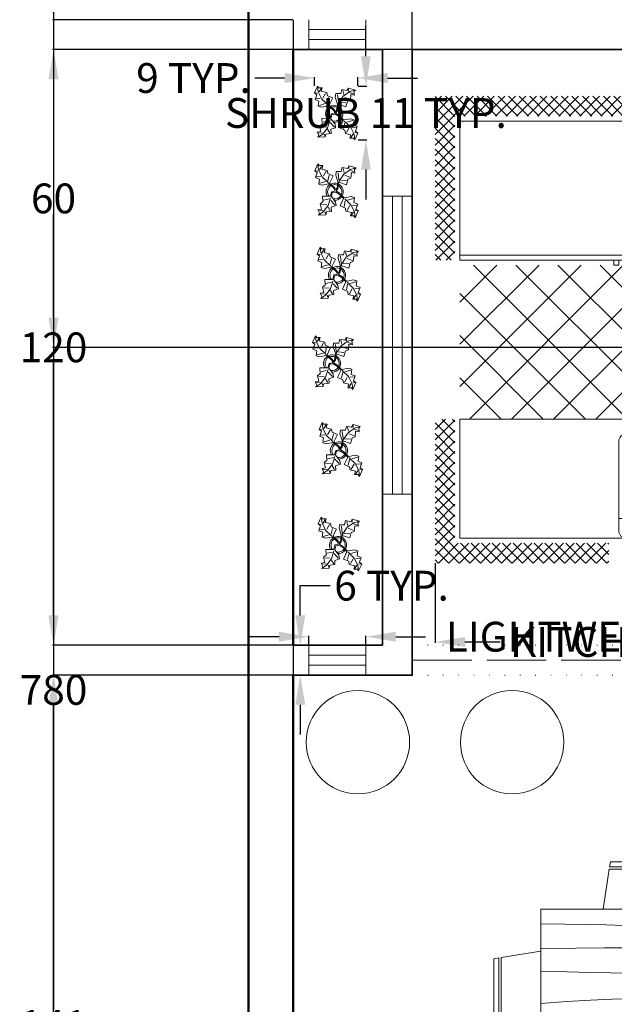
# Model space of a CAD drawing. Units: inches. Extents: x 823 to 1335, y 207 to 1074.
# Tile 3 of 6: x 823 to 943, y 577 to 776. Entities that reach past the tile are written whole.
import ezdxf

# ---------------------------------------------------------------- set-up
doc = ezdxf.new("R2010")
doc.units = ezdxf.units.IN
doc.header["$MEASUREMENT"] = 0
doc.linetypes.add('ACAD_ISO02W100', pattern=[15, 12, -3])
doc.linetypes.add('ACAD_ISO07W100', pattern=[3, 0, -3])
for name, color, linetype, lineweight in [('A-ANNO-DIMS', 2, 'Continuous', 18), ('A-GLAZ-HIDN', 211, 'ACAD_ISO02W100', 18), ('A-GLAZ-OVHD', 211, 'ACAD_ISO07W100', 18), ('furniture', 21, 'Continuous', 18), ('inner wall', 102, 'Continuous', 35), ('kitchen', 171, 'Continuous', 18), ('L-PLNT', 90, 'Continuous', 13), ('outer wall', 105, 'Continuous', 50), ('windows', 211, 'Continuous', 18)]:
    doc.layers.add(name, color=color, linetype=linetype, lineweight=lineweight)
doc.styles.get("Standard").update_dxf_attribs({"font": 'arial.ttf'})
doc.dimstyles.get("Standard").update_dxf_attribs({"dimtxt": 6, "dimasz": 6, "dimexe": 0.18, "dimexo": 0.0625, "dimgap": 0.09, "dimtad": 0, "dimtih": 1, "dimtoh": 1, "dimdec": 0, "dimzin": 0, "dimdsep": 46, "dimlunit": 3, "dimtxsty": 'Standard', "dimcen": 0.09, "dimadec": 0, "dimazin": 0, "dimtfac": 1, "dimtdec": 0, "dimtofl": 0, "dimtmove": 0, "dimatfit": 3, "dimfxl": 1, "dimtolj": 1, "dimtzin": 0, "dimarcsym": 0})

# ---------------------------------------------------------------- blocks, each defined once
blk = doc.blocks.new('Dining Set - 36 x 72 in.')
for p, q in [((-22.2343, 26.00059), (-23.4847, 17.99762)), ((-22.2304, 26), (-5.7608, 26)), ((-22, 27.5), (-22.1562, 26.50042)), ((-5.8416, 26.5), (-22.1534, 26.5)), ((-22, 27.5), (-6, 27.5)), ((-5.8437, 26.49966), (-6, 27.5)), ((-4.5152, 17.99762), (-5.7655, 25.99926)), ((5.7657, 26.00059), (4.5153, 17.99762)), ((5.7696, 26), (22.2392, 26)), ((6, 27.5), (5.8438, 26.50042)), ((22.1584, 26.5), (5.8466, 26.5)), ((6, 27.5), (22, 27.5)), ((22.1563, 26.49966), (22, 27.5)), ((23.4848, 17.99762), (22.2345, 25.99926)), ((36, 18), (-36, 18)), ((-36, 18), (-36, -18)), ((36, -18), (36, 18)), ((-45.5, 8), (-44.5004, 8.15617)), ((-45.5, 8), (-45.5, -8)), ((-44.5, -8.15843), (-44.5, 8.15338)), ((-44.0006, 8.23428), (-35.9976, 9.48474)), ((-44, 8.23041), (-44, -8.23915)), ((44.0006, 8.23428), (35.9976, 9.48474)), ((44, 8.23041), (44, -8.23915)), ((44.5, -8.15843), (44.5, 8.15338)), ((45.5, 8), (44.5005, 8.15617)), ((45.5, 8), (45.5, -8)), ((-44.4997, -8.15631), (-45.5, -8)), ((-35.9976, -9.48476), (-43.9993, -8.2345)), ((35.9976, -9.48476), (43.9993, -8.2345)), ((44.4997, -8.15631), (45.5, -8)), ((-36, -18), (36, -18)), ((-22.2343, -26.0006), (-23.4847, -17.99762)), ((-4.5152, -17.99762), (-5.7655, -25.99928)), ((5.7657, -26.0006), (4.5153, -17.99762)), ((23.4848, -17.99762), (22.2345, -25.99928)), ((-22.2304, -26), (-5.7608, -26)), ((-22, -27.5), (-22.1562, -26.50044)), ((-5.8416, -26.5), (-22.1534, -26.5)), ((-22, -27.5), (-6, -27.5)), ((-5.8437, -26.49967), (-6, -27.5)), ((5.7696, -26), (22.2392, -26)), ((6, -27.5), (5.8438, -26.50044)), ((22.1584, -26.5), (5.8466, -26.5)), ((6, -27.5), (22, -27.5)), ((22.1563, -26.49967), (22, -27.5))]:
    blk.add_line(p, q)
for points in [[(-36, 15), (-31.1772, 14.97754), (-26.8079, 14.91406), (-22.8538, 14.81543), (-19.276, 14.6875), (-16.0362, 14.53613), (-13.0957, 14.36718), (-10.4159, 14.18652), (-7.9583, 14), (-5.6904, 13.81315), (-3.6035, 13.63021), (-1.6954, 13.45508), (0.0365, 13.29166), (1.5945, 13.14388), (2.9811, 13.01562), (4.1988, 12.9108), (5.25, 12.83333), (6.1393, 12.78613), (6.8802, 12.76823), (7.4883, 12.77767), (7.9792, 12.8125), (8.3685, 12.87077), (8.6719, 12.95052), (8.9049, 13.0498), (9.0833, 13.16666), (9.2205, 13.29899), (9.3216, 13.44401), (9.3895, 13.59879), (9.4271, 13.76041), (9.4373, 13.92594), (9.4232, 14.09245), (9.3875, 14.257), (9.3333, 14.41666), (9.2638, 14.56917), (9.1836, 14.71484), (9.0975, 14.85465), (9.0104, 14.98958), (8.9272, 15.1206), (8.8529, 15.2487), (8.7922, 15.37483), (8.75, 15.5), (8.7305, 15.62467), (8.7344, 15.74739), (8.7617, 15.86621), (8.8125, 15.97916), (8.8867, 16.08431), (8.9844, 16.17968), (9.1055, 16.26334), (9.25, 16.33333), (9.4189, 16.38802), (9.6172, 16.42708), (9.8506, 16.45052), (10.125, 16.45833), (10.4463, 16.45052), (10.8203, 16.42708), (11.2529, 16.38802), (11.75, 16.33333), (12.3184, 16.26318), (12.9694, 16.17838), (13.7151, 16.07991), (14.5677, 15.96875), (15.5395, 15.84586), (16.6426, 15.71224), (17.8893, 15.56884), (19.2917, 15.41666), (20.859, 15.25667), (22.5879, 15.08984), (24.4721, 14.91715), (26.5052, 14.73958), (28.6809, 14.5581), (30.9929, 14.3737), (33.4347, 14.18733), (36, 14)], [(-36, 10), (-28.9766, 10.14274), (-23.1725, 10.20442), (-18.4241, 10.19775), (-14.5677, 10.13541), (-11.4399, 10.03011), (-8.877, 9.89453), (-6.7154, 9.74137), (-4.7917, 9.58333), (-2.9698, 9.43082), (-1.2246, 9.28515), (0.4415, 9.14534), (2.026, 9.01041), (3.5266, 8.87939), (4.9408, 8.7513), (6.266, 8.62516), (7.5, 8.5), (8.6411, 8.37549), (9.6914, 8.2539), (10.6538, 8.13818), (11.5312, 8.03125), (12.3267, 7.93603), (13.043, 7.85547), (13.6831, 7.79248), (14.25, 7.75), (14.7471, 7.7303), (15.1797, 7.73307), (15.5537, 7.75732), (15.875, 7.80208), (16.1494, 7.86637), (16.3828, 7.94922), (16.5811, 8.04964), (16.75, 8.16666), (16.8944, 8.29915), (17.0143, 8.44531), (17.1089, 8.60319), (17.1771, 8.77083), (17.218, 8.94629), (17.2305, 9.1276), (17.2137, 9.31282), (17.1667, 9.5), (17.0895, 9.6875), (16.987, 9.875), (16.8649, 10.0625), (16.7292, 10.25), (16.5856, 10.4375), (16.4401, 10.625), (16.2985, 10.8125), (16.1667, 11), (16.05, 11.18733), (15.9518, 11.3737), (15.8752, 11.5581), (15.8229, 11.73958), (15.798, 11.91715), (15.8034, 12.08984), (15.842, 12.25667), (15.9167, 12.41666), (16.0295, 12.56836), (16.1784, 12.70833), (16.3605, 12.83268), (16.5729, 12.9375), (16.8127, 13.01888), (17.0768, 13.07291), (17.3625, 13.0957), (17.6667, 13.08333), (17.9894, 13.03312), (18.3418, 12.94726), (18.7382, 12.82918), (19.1927, 12.68229), (19.7195, 12.51001), (20.3327, 12.31575), (21.0465, 12.10294), (21.875, 11.875), (22.8357, 11.63354), (23.959, 11.37304), (25.2786, 11.08618), (26.8282, 10.76562), (28.6414, 10.40405), (30.752, 9.99414), (33.1936, 9.52856), (36, 9)], [(-36, 5.5), (-30.7157, 5.3348), (-26.069, 5.20963), (-21.9946, 5.11767), (-18.4271, 5.05208), (-15.3009, 5.00602), (-12.5508, 4.97265), (-10.1112, 4.94515), (-7.9167, 4.91666), (-5.909, 4.88167), (-4.0586, 4.83984), (-2.3429, 4.79215), (-0.7396, 4.73958), (0.7739, 4.6831), (2.22, 4.6237), (3.6213, 4.56233), (5, 4.5), (6.373, 4.43782), (7.7344, 4.3776), (9.0723, 4.32129), (10.375, 4.27083), (11.6309, 4.22819), (12.8281, 4.19531), (13.9551, 4.17415), (15, 4.16666), (15.954, 4.17448), (16.819, 4.19791), (17.6001, 4.23698), (18.3021, 4.29166), (18.9299, 4.36198), (19.4883, 4.44791), (19.9823, 4.54948), (20.4167, 4.66666), (20.7969, 4.79899), (21.1302, 4.94401), (21.4245, 5.09879), (21.6875, 5.26041), (21.9271, 5.42594), (22.1511, 5.59245), (22.3672, 5.757), (22.5834, 5.91666), (22.8065, 6.06868), (23.0404, 6.21093), (23.2879, 6.34147), (23.5521, 6.45833), (23.8358, 6.55957), (24.142, 6.64323), (24.4735, 6.70735), (24.8334, 6.75), (25.2235, 6.76969), (25.642, 6.76692), (26.0858, 6.74267), (26.5521, 6.69791), (27.0379, 6.63362), (27.5404, 6.55078), (28.0565, 6.45036), (28.5834, 6.33333), (29.1242, 6.19987), (29.7071, 6.04687), (30.3661, 5.87044), (31.1354, 5.66666), (32.0493, 5.43164), (33.142, 5.16146), (34.4475, 4.85221), (36, 4.5)], [(-36, -1), (-30.7915, -0.6591), (-26.0195, -0.38216), (-21.6519, -0.16284), (-17.6563, 0.00521), (-14.0005, 0.12833), (-10.6523, 0.21289), (-7.5796, 0.26522), (-4.75, 0.29166), (-2.134, 0.29793), (0.2878, 0.28711), (2.5317, 0.26163), (4.6146, 0.22396), (6.5529, 0.17651), (8.3633, 0.12174), (10.0623, 0.06209), (11.6667, 0), (13.1899, -0.06201), (14.6341, -0.1211), (15.9982, -0.17432), (17.2813, -0.21875), (18.4823, -0.25147), (19.6003, -0.26953), (20.6343, -0.27002), (21.5834, -0.25), (22.4481, -0.20768), (23.2357, -0.14584), (23.9549, -0.06836), (24.6146, 0.02083), (25.2235, 0.11784), (25.7904, 0.21875), (26.3241, 0.31966), (26.8334, 0.41666), (27.3265, 0.50618), (27.8099, 0.58593), (28.2894, 0.65397), (28.7709, 0.70833), (29.2601, 0.74707), (29.763, 0.76823), (30.2855, 0.76985), (30.8334, 0.75), (31.4088, 0.70784), (31.9994, 0.64713), (32.589, 0.57275), (33.1615, 0.48958), (33.7008, 0.4025), (34.1908, 0.3164), (34.6153, 0.23616), (34.9584, 0.16666), (35.2099, 0.11165), (35.3848, 0.07031), (35.504, 0.04069), (35.5886, 0.02083), (35.6594, 0.00879), (35.7377, 0.0026), (35.8442, 0.00032), (36, 0)], [(-36, -6.5), (-27.1843, -6.31267), (-20.084, -6.1263), (-14.469, -5.9419), (-10.1094, -5.76042), (-6.7752, -5.58285), (-4.2363, -5.41016), (-2.2629, -5.24333), (-0.625, -5.08334), (0.8708, -4.93099), (2.2715, -4.78646), (3.5872, -4.64974), (4.8281, -4.52084), (6.0046, -4.39974), (7.127, -4.28646), (8.2053, -4.18099), (9.25, -4.08334), (10.2705, -3.99382), (11.2734, -3.91407), (12.2647, -3.84603), (13.25, -3.79167), (14.2354, -3.75293), (15.2266, -3.73177), (16.2295, -3.73015), (17.25, -3.75), (18.2912, -3.79248), (19.3451, -3.85547), (20.4009, -3.93604), (21.4479, -4.03125), (22.4754, -4.13819), (23.4727, -4.25391), (24.4289, -4.37549), (25.3334, -4.5), (26.1785, -4.62492), (26.9694, -4.74935), (27.7145, -4.87281), (28.4219, -4.99479), (29.1, -5.11483), (29.7572, -5.23242), (30.4016, -5.34709), (31.0417, -5.45834), (31.6837, -5.56437), (32.3262, -5.65821), (32.9658, -5.73153), (33.599, -5.77604), (34.2224, -5.78345), (34.8327, -5.74545), (35.4264, -5.65373), (36, -5.5)], [(-36, -10), (-26.4022, -9.81299), (-18.4675, -9.62891), (-11.9839, -9.45069), (-6.7396, -9.28125), (-2.5226, -9.12354), (0.8789, -8.98047), (3.6769, -8.85498), (6.0833, -8.75), (8.2767, -8.66765), (10.3021, -8.60677), (12.1712, -8.56543), (13.8958, -8.54167), (15.4876, -8.53353), (16.9583, -8.53907), (18.3197, -8.55632), (19.5834, -8.58334), (20.7616, -8.61841), (21.8685, -8.66081), (22.9188, -8.71004), (23.9271, -8.76563), (24.9081, -8.82707), (25.8763, -8.89388), (26.8465, -8.96558), (27.8334, -9.04167), (28.8474, -9.12118), (29.8828, -9.20117), (30.93, -9.27824), (31.9792, -9.34896), (33.0205, -9.40991), (34.0443, -9.45768), (35.0407, -9.48885), (36, -9.5)], [(-36, -14.5), (-30.0881, -14.33513), (-25.0332, -14.21224), (-20.7312, -14.12647), (-17.0781, -14.07292), (-13.97, -14.04671), (-11.3027, -14.04297), (-8.9724, -14.05681), (-6.875, -14.08334), (-4.9224, -14.11833), (-3.0905, -14.16016), (-1.3709, -14.20785), (0.2448, -14.26042), (1.7647, -14.3169), (3.1973, -14.3763), (4.5507, -14.43767), (5.8333, -14.5), (7.0554, -14.5621), (8.235, -14.62175), (9.3922, -14.67652), (10.5469, -14.72396), (11.7192, -14.76164), (12.929, -14.78711), (14.1965, -14.79794), (15.5417, -14.79167), (16.9933, -14.76424), (18.6152, -14.70508), (20.4804, -14.60197), (22.6615, -14.44271), (25.2312, -14.21509), (28.2624, -13.9069), (31.8277, -13.50594), (36, -13)]]:
    blk.add_lwpolyline(points)
blk = doc.blocks.new('Kitchen Layout - 7 x 8 ft')
for p, q in [((-5, 81.32), (2.68, 89)), ((-5, 83.44), (0.56, 89)), ((-5, 85.56), (-1.56, 89)), ((-5, 87.68), (-3.68, 89)), ((-1, 84.97), (-5, 88.97)), ((1.09, 85), (-2.91, 89)), ((3.21, 85), (-0.79, 89)), ((0.81, 85), (4.81, 89)), ((5.34, 85), (1.34, 89)), ((2.93, 85), (6.93, 89)), ((7.46, 85), (3.46, 89)), ((5.05, 85), (9.05, 89)), ((9.58, 85), (5.58, 89)), ((7.17, 85), (11.17, 89)), ((11.7, 85), (7.7, 89)), ((9.29, 85), (13.29, 89)), ((13.82, 85), (9.82, 89)), ((11.41, 85), (15.41, 89)), ((15.94, 85), (11.94, 89)), ((13.53, 85), (17.53, 89)), ((18.06, 85), (14.06, 89)), ((15.65, 85), (19.65, 89)), ((20.18, 85), (16.18, 89)), ((17.78, 85), (21.78, 89)), ((22.31, 85), (18.31, 89)), ((19.9, 85), (23.9, 89)), ((24.43, 85), (20.43, 89)), ((22.02, 85), (26.02, 89)), ((26.55, 85), (22.55, 89)), ((24.14, 85), (28.14, 89)), ((28.67, 85), (24.67, 89)), ((26.26, 85), (30.26, 89)), ((30.79, 85), (26.79, 89)), ((28.38, 85), (32.38, 89)), ((32.91, 85), (28.91, 89)), ((30.5, 85), (34.5, 89)), ((35.03, 85), (31.03, 89)), ((32.63, 85), (36.63, 89)), ((37.16, 85), (33.16, 89)), ((34.75, 85), (38.75, 89)), ((39.28, 85), (35.28, 89)), ((36.87, 85), (40.87, 89)), ((41.4, 85), (37.4, 89)), ((38.99, 85), (42.99, 89)), ((43.52, 85), (39.52, 89)), ((41.11, 85), (45.11, 89)), ((45.64, 85), (41.64, 89)), ((43.23, 85), (47.23, 89)), ((47.76, 85), (43.76, 89)), ((45.35, 85), (49.35, 89)), ((49.88, 85), (45.88, 89)), ((47.47, 85), (51.47, 89)), ((52, 85), (48, 89)), ((49.6, 85), (53.6, 89)), ((54.13, 85), (50.13, 89)), ((51.72, 85), (55.72, 89)), ((56.25, 85), (52.25, 89)), ((53.84, 85), (57.84, 89)), ((58.37, 85), (54.37, 89)), ((55.96, 85), (59.96, 89)), ((60.49, 85), (56.49, 89)), ((58.08, 85), (62.08, 89)), ((62.61, 85), (58.61, 89)), ((60.2, 85), (64.2, 89)), ((64.73, 85), (60.73, 89)), ((62.32, 85), (66.32, 89)), ((66.85, 85), (62.85, 89)), ((64.45, 85), (68.45, 89)), ((68.97, 85), (64.97, 89)), ((66.57, 85), (70.57, 89)), ((71.1, 85), (67.1, 89)), ((68.69, 85), (72.69, 89)), ((73.22, 85), (69.22, 89)), ((70.81, 85), (74.81, 89)), ((75.34, 85), (71.34, 89)), ((72.93, 85), (76.93, 89)), ((77.46, 85), (73.46, 89)), ((75.05, 85), (79.05, 89)), ((79.58, 85), (75.58, 89)), ((77.17, 85), (81.17, 89)), ((81.7, 85), (77.7, 89)), ((79.29, 85), (83.29, 89)), ((83.82, 85), (79.82, 89)), ((81.42, 85), (85.42, 89)), ((85.95, 85), (81.95, 89)), ((83.54, 85), (87.54, 89)), ((88.07, 85), (84.07, 89)), ((85.66, 85), (89.66, 89)), ((90.19, 85), (86.19, 89)), ((87.78, 85), (91.78, 89)), ((92.31, 85), (88.31, 89)), ((89.9, 85), (93.9, 89)), ((94.43, 85), (90.43, 89)), ((92.02, 85), (96.02, 89)), ((96.55, 85), (92.55, 89)), ((94.14, 85), (98.14, 89)), ((101, 82.67), (94.67, 89)), ((96.27, 85), (100.27, 89)), ((101, 84.79), (96.79, 89)), ((97, 83.61), (101, 87.61)), ((101, 86.92), (98.92, 89)), ((-1, 82.85), (-5, 86.85)), ((97, 81.49), (101, 85.49)), ((-1, 80.73), (-5, 84.73)), ((34, 84), (96, 84)), ((34, 60), (34, 84)), ((96, 84), (96, 60)), ((101, 80.55), (97, 84.55)), ((97, 79.37), (101, 83.37)), ((-5, 79.19), (-1, 83.19)), ((-1, 78.61), (-5, 82.61)), ((101, 78.43), (97, 82.43)), ((-5, 77.07), (-1, 81.07)), ((-1, 76.49), (-5, 80.49)), ((74, 81), (95, 81)), ((97, 77.25), (101, 81.25)), ((101, 76.31), (97, 80.31)), ((-5, 74.95), (-1, 78.95)), ((-1, 74.36), (-5, 78.36)), ((97, 75.13), (101, 79.13)), ((101, 74.19), (97, 78.19)), ((-5, 72.83), (-1, 76.83)), ((-1, 72.24), (-5, 76.24)), ((97, 73.01), (101, 77.01)), ((101, 72.07), (97, 76.07)), ((-5, 70.71), (-1, 74.71)), ((-1, 70.12), (-5, 74.12)), ((97, 70.89), (101, 74.89)), ((101, 69.95), (97, 73.95)), ((-5, 68.59), (-1, 72.59)), ((-1, 68), (-5, 72)), ((97, 68.76), (101, 72.76)), ((101, 67.82), (97, 71.82)), ((-5, 66.47), (-1, 70.47)), ((-1, 65.88), (-5, 69.88)), ((97, 66.64), (101, 70.64)), ((101, 65.7), (97, 69.7)), ((-5, 64.35), (-1, 68.35)), ((-1, 63.76), (-5, 67.76)), ((97, 64.52), (101, 68.52)), ((101, 63.58), (97, 67.58)), ((-5, 62.22), (-1, 66.22)), ((-1, 61.64), (-5, 65.64)), ((97, 62.4), (101, 66.4)), ((101, 61.46), (97, 65.46)), ((-5, 60.1), (-1, 64.1)), ((-1, 59.52), (-5, 63.52)), ((97, 60.28), (101, 64.28)), ((-5, 57.98), (-1, 61.98)), ((100.34, 60), (97, 63.34)), ((98.84, 60), (101, 62.16)), ((-1, 57.39), (-5, 61.39)), ((-4.86, 56), (-1, 59.86)), ((10.4, 24), (45.9, 59.5)), ((18.88, 24), (54.38, 59.5)), ((27.37, 24), (62.87, 59.5)), ((33.03, 55.11), (37.41, 59.5)), ((96, 60), (34, 60)), ((35.85, 24), (71.35, 59.5)), ((76.2, 24), (40.7, 59.5)), ((84.68, 24), (49.18, 59.5)), ((93.17, 24), (57.67, 59.5)), ((96, 29.65), (66.15, 59.5)), ((80, 60), (80, 59)), ((82, 59), (82, 60)), ((87, 59), (87, 60)), ((89, 60), (89, 59)), ((98.22, 60), (97, 61.22)), ((100.96, 60), (101, 60.04)), ((-1.73, 56), (-5, 59.27)), ((-2.74, 56), (-1, 57.74)), ((67.71, 24), (33.68, 58.04)), ((61.31, 24), (96, 58.69)), ((96, 55.11), (93.57, 57.54)), ((-3.85, 56), (-5, 57.15)), ((0, 57), (33, 57)), ((31, 55), (31, 56)), ((32, 56), (32, 55)), ((44.34, 24), (77.84, 57.5)), ((52.82, 24), (86.32, 57.5)), ((96, 38.14), (76.64, 57.5)), ((96, 46.63), (85.13, 57.5)), ((0, 30.57), (24.43, 55)), ((0, 39.06), (15.94, 55)), ((0, 47.54), (7.46, 55)), ((1.91, 24), (32.91, 55)), ((33.77, 24), (2.77, 55)), ((42.26, 24), (11.26, 55)), ((50.74, 24), (19.74, 55)), ((59.23, 24), (28.23, 55)), ((32, 55), (31, 55)), ((69.79, 24), (96, 50.21)), ((25.29, 24), (0, 49.29)), ((78.28, 24), (96, 41.72)), ((16.8, 24), (0, 40.8)), ((8.32, 24), (0, 32.32)), ((86.76, 24), (96, 33.24)), ((-5, 21.92), (-2.92, 24)), ((-1, 21.33), (-3.67, 24)), ((-1, 23.45), (-1.55, 24)), ((0, 24), (96, 24)), ((0, 0), (0, 24)), ((95.25, 24), (96, 24.75)), ((96, 24), (96, 0)), ((97, 22.1), (98.9, 24)), ((97, 19.97), (101, 23.97)), ((101, 21.16), (98.16, 24)), ((101, 23.28), (100.28, 24)), ((-5, 19.8), (-1, 23.8)), ((-1, 19.21), (-5, 23.21)), ((101, 19.03), (97, 23.03)), ((97, 17.85), (101, 21.85)), ((-5, 17.68), (-1, 21.68)), ((-1, 17.09), (-5, 21.09)), ((101, 16.91), (97, 20.91)), ((-5, 15.55), (-1, 19.55)), ((-1, 14.97), (-5, 18.97)), ((47.25, 6.5), (47.25, 18.5)), ((48.75, 18.5), (48.75, 6.5)), ((97, 15.73), (101, 19.73)), ((101, 14.79), (97, 18.79)), ((-5, 13.43), (-1, 17.43)), ((-1, 12.85), (-5, 16.85)), ((97, 13.61), (101, 17.61)), ((101, 12.67), (97, 16.67)), ((-5, 11.31), (-1, 15.31)), ((-1, 10.73), (-5, 14.73)), ((97, 11.49), (101, 15.49)), ((101, 10.55), (97, 14.55)), ((-5, 9.19), (-1, 13.19)), ((-1, 8.6), (-5, 12.6)), ((97, 9.37), (101, 13.37)), ((101, 8.43), (97, 12.43)), ((-5, 7.07), (-1, 11.07)), ((-1, 6.48), (-5, 10.48)), ((97, 7.25), (101, 11.25)), ((101, 6.31), (97, 10.31)), ((-5, 4.95), (-1, 8.95)), ((-1, 4.36), (-5, 8.36)), ((97, 5.12), (101, 9.12)), ((101, 4.18), (97, 8.18)), ((-5, 2.83), (-1, 6.83)), ((-1, 2.24), (-5, 6.24)), ((97, 3), (101, 7)), ((101, 2.06), (97, 6.06)), ((-5, 0.71), (-1, 4.71)), ((-1, 0.12), (-5, 4.12)), ((64, 4), (32, 4)), ((97, 0.88), (101, 4.88)), ((-5, -1.42), (-1, 2.58)), ((2, -5), (-5, 2)), ((93.24, -5), (101, 2.76)), ((101, -0.06), (97, 3.94)), ((-5, -3.54), (-1, 0.46)), ((96, 0), (0, 0)), ((95.36, -5), (101, 0.64)), ((101, -2.18), (97, 1.82)), ((-0.12, -5), (-5, -0.12)), ((-4.34, -5), (-0.34, -1)), ((-2.22, -5), (1.78, -1)), ((-0.1, -5), (3.9, -1)), ((4.12, -5), (0.12, -1)), ((2.02, -5), (6.02, -1)), ((6.24, -5), (2.24, -1)), ((4.14, -5), (8.14, -1)), ((8.36, -5), (4.36, -1)), ((6.27, -5), (10.27, -1)), ((10.48, -5), (6.48, -1)), ((8.39, -5), (12.39, -1)), ((12.6, -5), (8.6, -1)), ((10.51, -5), (14.51, -1)), ((14.73, -5), (10.73, -1)), ((12.63, -5), (16.63, -1)), ((16.85, -5), (12.85, -1)), ((14.75, -5), (18.75, -1)), ((18.97, -5), (14.97, -1)), ((16.87, -5), (20.87, -1)), ((21.09, -5), (17.09, -1)), ((18.99, -5), (22.99, -1)), ((23.21, -5), (19.21, -1)), ((21.11, -5), (25.11, -1)), ((25.33, -5), (21.33, -1)), ((23.24, -5), (27.24, -1)), ((27.45, -5), (23.45, -1)), ((25.36, -5), (29.36, -1)), ((29.57, -5), (25.57, -1)), ((30, -3.3), (27.7, -1)), ((30, -1.18), (29.82, -1)), ((66, -2.54), (67.54, -1)), ((66, -4.66), (69.66, -1)), ((69.88, -5), (66, -1.12)), ((67.78, -5), (71.78, -1)), ((72, -5), (68, -1)), ((69.9, -5), (73.9, -1)), ((74.12, -5), (70.12, -1)), ((72.03, -5), (76.03, -1)), ((76.24, -5), (72.24, -1)), ((74.15, -5), (78.15, -1)), ((78.36, -5), (74.36, -1)), ((76.27, -5), (80.27, -1)), ((80.49, -5), (76.49, -1)), ((78.39, -5), (82.39, -1)), ((82.61, -5), (78.61, -1)), ((80.51, -5), (84.51, -1)), ((84.73, -5), (80.73, -1)), ((82.63, -5), (86.63, -1)), ((86.85, -5), (82.85, -1)), ((84.75, -5), (88.75, -1)), ((88.97, -5), (84.97, -1)), ((86.88, -5), (90.88, -1)), ((91.09, -5), (87.09, -1)), ((89, -5), (93, -1)), ((93.21, -5), (89.21, -1)), ((91.12, -5), (95.12, -1)), ((95.34, -5), (91.34, -1)), ((97.46, -5), (93.46, -1)), ((99.58, -5), (95.58, -1)), ((101, -4.3), (97, -0.3)), ((97.48, -5), (101, -1.48)), ((-2.25, -5), (-5, -2.25)), ((27.48, -5), (30, -2.48)), ((67.76, -5), (66, -3.24)), ((99.6, -5), (101, -3.6)), ((-4.37, -5), (-5, -4.37)), ((29.6, -5), (30, -4.6))]:
    blk.add_line(p, q)
for points in [[(0, 56), (0, 84), (33, 84), (33, 56)], [(74, 60), (74, 84), (95, 84), (95, 60)], [(76, 58), (76, 59), (93, 59), (93, 58)]]:
    blk.add_lwpolyline(points, close=True)
for points in [[(33.5, 21), (62.5, 21)], [(32, 1.5), (32, 19.5)], [(33.5, 6.5), (33.5, 18.5)], [(34.5, 19.5), (46.25, 19.5)], [(49.75, 19.5), (61.5, 19.5)], [(62.5, 18.5), (62.5, 6.5)], [(64, 19.5), (64, 1.5)], [(46.25, 5.5), (34.5, 5.5)], [(61.5, 5.5), (49.75, 5.5)], [(62.5, 0), (33.5, 0)]]:
    blk.add_lwpolyline(points)
for centre, radius in [((80, 75), 4), ((80, 75), 3), ((89, 75), 3), ((80, 75), 2), ((80, 75), 1), ((89, 75), 2), ((89, 75), 1), ((89, 66), 4), ((80, 66), 3), ((80, 66), 2), ((89, 66), 3), ((89, 66), 2), ((80, 66), 1), ((89, 66), 1), ((40.5, 12.5), 1), ((40.5, 12.5), 0.5), ((55.5, 12.5), 1), ((55.5, 12.5), 0.5)]:
    blk.add_circle(centre, radius)
for centre, radius, start, end in [((33.5, 19.5), 1.5, 90, 180), ((62.5, 19.5), 1.5, 0, 90), ((34.5, 18.5), 1, 90, 180), ((46.25, 18.5), 1, 0, 90), ((49.75, 18.5), 1, 90, 180), ((61.5, 18.5), 1, 0, 90), ((34.5, 6.5), 1, 180, 270), ((46.25, 6.5), 1, 270, 0), ((49.75, 6.5), 1, 180, 270), ((61.5, 6.5), 1, 270, 0), ((33.5, 1.5), 1.5, 180, 270), ((62.5, 1.5), 1.5, 270, 0)]:
    blk.add_arc(centre, radius, start, end)
blk = doc.blocks.new('Plant - Rubber or Philodendron')
for p, q in [((13.3837, 12.301), (14.68, 13.9039)), ((14.68, 13.9039), (19.3848, 11.8146)), ((-16.2005, 11.4774), (-13.9899, 8.1064)), ((-16.2005, 11.4774), (-14.8639, 10.7964)), ((-16.0159, 6.3329), (-16.2005, 11.4774)), ((-15.3434, 6.5514), (-13.9984, 6.9884)), ((-14.8639, 10.7964), (-12.6195, 11.8975)), ((-13.9899, 8.1064), (-9.5434, 4.7185)), ((-13.3174, 8.325), (-13.0735, 11.0065)), ((-12.6195, 11.8975), (-12.1909, 9.4345)), ((-12.1909, 9.4345), (-8.3829, 10.3)), ((-8.8369, 9.409), (-9.0894, 5.6095)), ((-8.3829, 10.3), (-7.0549, 8.501)), ((-7.0549, 8.501), (-3.0284, 8.6941)), ((-4.8529, 4.012), (-5.7184, 7.82)), ((-3.0284, 8.6941), (-3.0709, 3.1041)), ((4.6914, 8.8812), (5.3859, 11.2828)), ((4.6914, 8.8812), (5.5014, 4.4831)), ((5.3859, 11.2828), (8.8871, 10.7908)), ((5.9878, 10.4842), (7.1971, 6.3869)), ((10.3916, 8.7942), (6.2847, 4.4028)), ((8.8871, 10.7908), (9.9809, 13.4933)), ((9.9809, 13.4933), (13.3837, 12.301)), ((15.3859, 11.3055), (10.3916, 8.7942)), ((10.5828, 12.6946), (10.8893, 9.7953)), ((14.2977, 6.1031), (10.9934, 7.9956)), ((14.5816, 13.2037), (14.3848, 11.8033)), ((15.7909, 9.1065), (14.8995, 5.3044)), ((15.2875, 10.6053), (17.5907, 9.2105)), ((19.3848, 11.8146), (15.3859, 11.3055)), ((18.1925, 8.4119), (15.7909, 9.1065)), ((19.3848, 11.8146), (18.1868, 10.9119)), ((18.1868, 10.9119), (18.1925, 8.4119)), ((-14.0069, 5.8704), (-16.0159, 6.3329)), ((-13.5868, 2.2894), (-14.0069, 5.8704)), ((-10.6784, 2.491), (-13.5868, 2.2894)), ((-13.1329, 3.1804), (-10.6614, 4.727)), ((-9.5858, -0.8715), (-10.6784, 2.491)), ((-9.5434, 4.7185), (-4.1917, 2.9888)), ((-9.1318, 0.0195), (-5.9793, 2.9025)), ((-7.1228, -0.443), (-3.5248, 2.2131)), ((-3.5248, 2.2131), (-3.3011, 2.4355)), ((-3.3011, 2.4355), (-0.5306, 1.7947)), ((-3.0709, 3.1041), (0.0797, 2.3163)), ((-0.5306, 1.7947), (-0.2255, -0.5527)), ((-0.5306, 1.7947), (-0.5306, 1.7947)), ((0.0797, 2.3163), (0.4866, -0.031)), ((0.4866, -0.031), (2.1141, 0.2298)), ((2.1141, 0.2298), (5.4346, 3.9146)), ((6.1032, 3.6844), (2.8262, -0.031)), ((5.4346, 3.9146), (5.5014, 4.4831)), ((11.1089, 1.1958), (6.1032, 3.6844)), ((7.7005, 4.8881), (11.5025, 3.9967)), ((12.7005, 4.8994), (11.1089, 1.1958)), ((14.8995, 5.3044), (12.7005, 4.8994)), ((-11.3237, -7.2629), (-9.7321, -3.5593)), ((-6.3237, -7.2516), (-10.1257, -6.3602)), ((-9.7321, -3.5593), (-4.7264, -6.0479)), ((-7.1228, -0.443), (-9.5858, -0.8715)), ((-9.0148, -11.1577), (-4.9047, -6.8122)), ((-2.019, -3.6148), (-4.7264, -6.0479)), ((-4.1246, -6.8466), (-4.0579, -6.2781)), ((-3.3146, -11.2447), (-4.1246, -6.8466)), ((-4.0579, -6.2781), (-0.9375, -3.1608)), ((-2.019, -3.6148), (-0.2255, -0.5527)), ((-0.9375, -3.1608), (0.5883, -0.8135)), ((0.5883, -0.8135), (2.2447, -2.0916)), ((2.8262, -0.031), (1.3003, -0.5527)), ((1.3003, -0.5527), (2.4193, -1.4655)), ((2.2447, -2.0916), (6.7108, -2.6626)), ((2.4193, -1.4655), (6.895, -2.1175)), ((4.943, -7.9659), (6.7108, -2.6626)), ((11.6605, -0.5413), (6.895, -2.1175)), ((12.3677, -6.1981), (7.219, -2.6772)), ((8.125, -4.0768), (7.7715, -7.9659)), ((8.3544, -2.7453), (13.1973, -2.1704)), ((11.6605, -0.5413), (14.1354, -0.8948)), ((15.5496, -10.7943), (12.3677, -6.1981)), ((16.2567, -5.8446), (13.4283, -6.5517)), ((14.1354, -0.8948), (14.1354, -4.4304)), ((14.1354, -4.4304), (16.9638, -5.1375)), ((16.9638, -5.1375), (16.2567, -8.673)), ((-18.008, -14.1781), (-16.8101, -13.2754)), ((-18.008, -14.1781), (-14.0091, -13.669)), ((-16.8157, -10.7754), (-14.4141, -11.4699)), ((-16.8101, -13.2754), (-16.8157, -10.7754)), ((-13.9107, -12.9688), (-16.2139, -11.574)), ((-14.4141, -11.4699), (-13.5228, -7.6679)), ((-14.0091, -13.669), (-9.0148, -11.1577)), ((-13.5228, -7.6679), (-11.3237, -7.2629)), ((-12.921, -8.4665), (-9.6166, -10.359)), ((-9.206, -15.0581), (-9.5126, -12.1588)), ((-7.5103, -13.1543), (-8.6042, -15.8568)), ((-4.0092, -13.6463), (-7.5103, -13.1543)), ((-4.611, -12.8477), (-5.8203, -8.7504)), ((-3.3146, -11.2447), (-4.0092, -13.6463)), ((8.8321, -9.0266), (4.943, -7.9659)), ((9.5392, -11.1479), (8.8321, -9.0266)), ((13.4283, -11.5015), (9.5392, -11.1479)), ((10.2463, -10.4408), (11.6605, -6.9053)), ((13.0748, -13.9763), (13.4283, -11.5015)), ((15.5496, -13.6228), (13.0748, -13.9763)), ((14.8425, -10.7943), (13.7819, -13.2692)), ((16.6103, -14.6834), (15.5496, -10.7943)), ((16.6103, -14.6834), (15.5496, -13.6228)), ((17.3174, -9.7337), (15.9032, -9.7337)), ((16.2567, -8.673), (18.0245, -9.7337)), ((18.0245, -9.7337), (16.6103, -14.6834)), ((-13.3032, -16.2674), (-18.008, -14.1781)), ((-12.0069, -14.6645), (-13.3032, -16.2674)), ((-13.2048, -15.5672), (-13.008, -14.1668)), ((-8.6042, -15.8568), (-12.0069, -14.6645))]:
    blk.add_line(p, q)
for centre, radius, start, end in [((0.0308, 0.1664), 6, 178.6147, 235.1169), ((0.0308, 0.1664), 5, 168.1647, 238.6725), ((0, 0), 6.1275, 34.37569, 120.1028), ((-0.0601, -0.2075), 5.2461, 33.82192, 124.9414), ((-0.2664, 0.1682), 5.2775, 338.4094, 20.03007), ((-0.098, 0.1364), 6.1288, 341.2017, 26.09184), ((-0.0234, 0.3825), 6.1492, 242.5812, 331.2714), ((-0.1102, 0.4886), 5.2883, 247.3711, 327.472)]:
    blk.add_arc(centre, radius, start, end)
blk = doc.blocks.new('WIN-60IN')
for p, q in [((0, 0), (0, 60)), ((0, 60), (6, 60)), ((2, 0), (2, 60)), ((4, 60), (4, 0)), ((6, 60), (6, 0)), ((6, 0), (0, 0))]:
    blk.add_line(p, q)
blk = doc.blocks.new('WIN-LIGHTWELL-NARROW')
for p, q in [((0, 6), (0, 0)), ((11.5, 6), (11.5, 0)), ((0, 4), (11.5, 4)), ((0, 2), (11.5, 2))]:
    blk.add_line(p, q)
blk = doc.blocks.new('STOOL-COUNTER-ROUND')
blk.add_circle((10.41, 10.41), 10.41)
blk = doc.blocks.new('*D32')
at = {"layer": 'A-ANNO-DIMS', "color": 0, "lineweight": -2, "transparency": 16777216}
for p, q in [((906.87, 666.11), (906.87, 650.09)), ((1012.87, 666.11), (1012.87, 650.09)), ((912.87, 650.27), (919.99, 650.27)), ((1006.87, 650.27), (999.75, 650.27))]:
    blk.add_line(p, q, dxfattribs=at)
for points in [[(912.87, 651.27), (912.87, 649.27), (906.87, 650.27)], [(1006.87, 651.27), (1006.87, 649.27), (1012.87, 650.27)]]:
    blk.add_solid(points, dxfattribs=at)
at = {"layer": 'Defpoints', "color": 0, "lineweight": -2, "transparency": 16777216}
for p in [(906.87, 666.17), (1012.87, 666.17), (1012.87, 650.27)]:
    blk.add_point(p, dxfattribs=at)
at = {"layer": 'A-ANNO-DIMS', "color": 0, "transparency": 16777216, "insert": (959.87, 650.27), "char_height": 6, "attachment_point": 5}
blk.add_mtext('\\A1;KITCHEN UNITS 106', dxfattribs=at)
blk = doc.blocks.new('*D50')
at = {"layer": 'A-ANNO-DIMS', "color": 0, "lineweight": -2, "transparency": 16777216}
for p, q in [((875.44, 651.33), (869.44, 651.33)), ((881.44, 649.67), (881.44, 651.51)), ((892.95, 649.67), (892.95, 651.51)), ((898.95, 651.33), (904.95, 651.33))]:
    blk.add_line(p, q, dxfattribs=at)
for points in [[(875.44, 652.33), (875.44, 650.33), (881.44, 651.33)], [(898.95, 652.33), (898.95, 650.33), (892.95, 651.33)]]:
    blk.add_solid(points, dxfattribs=at)
at = {"layer": 'Defpoints', "color": 0, "lineweight": -2, "transparency": 16777216}
for p in [(892.95, 651.33), (881.44, 649.61), (892.95, 649.61)]:
    blk.add_point(p, dxfattribs=at)
at = {"layer": 'A-ANNO-DIMS', "color": 0, "transparency": 16777216, "insert": (963.98, 651.33), "char_height": 6, "attachment_point": 5}
blk.add_mtext('\\A1;LIGHTWELL WINDOW 12 TYP.', dxfattribs=at)
blk = doc.blocks.new('*D51')
at = {"layer": 'A-ANNO-DIMS', "color": 0, "lineweight": -2, "transparency": 16777216}
for p, q in [((879.72, 655.61), (879.72, 661.61)), ((879.72, 661.61), (885.72, 661.61)), ((881.38, 649.61), (879.54, 649.61)), ((881.38, 643.61), (879.54, 643.61)), ((879.72, 637.61), (879.72, 631.61))]:
    blk.add_line(p, q, dxfattribs=at)
for points in [[(878.72, 655.61), (880.72, 655.61), (879.72, 649.61)], [(878.72, 637.61), (880.72, 637.61), (879.72, 643.61)]]:
    blk.add_solid(points, dxfattribs=at)
at = {"layer": 'Defpoints', "color": 0, "lineweight": -2, "transparency": 16777216}
for p in [(879.72, 649.61), (881.44, 649.61), (881.44, 643.61)]:
    blk.add_point(p, dxfattribs=at)
at = {"layer": 'A-ANNO-DIMS', "color": 0, "transparency": 16777216, "insert": (898.1, 661.61), "char_height": 6, "attachment_point": 5}
blk.add_mtext('\\A1;6 TYP.', dxfattribs=at)
blk = doc.blocks.new('*D54')
at = {"layer": 'A-ANNO-DIMS', "color": 0, "lineweight": -2, "transparency": 16777216}
for p, q in [((892.93, 768.23), (892.93, 774.23)), ((891.37, 762.23), (893.11, 762.23)), ((891.37, 751.4), (893.11, 751.4)), ((892.93, 745.4), (892.93, 739.4))]:
    blk.add_line(p, q, dxfattribs=at)
for points in [[(891.93, 768.23), (893.93, 768.23), (892.93, 762.23)], [(891.93, 745.4), (893.93, 745.4), (892.93, 751.4)]]:
    blk.add_solid(points, dxfattribs=at)
at = {"layer": 'Defpoints', "color": 0, "lineweight": -2, "transparency": 16777216}
for p in [(891.3, 762.23), (892.93, 762.23), (891.3, 751.4)]:
    blk.add_point(p, dxfattribs=at)
at = {"layer": 'A-ANNO-DIMS', "color": 0, "transparency": 16777216, "insert": (892.93, 756.82), "char_height": 6, "attachment_point": 5}
blk.add_mtext('\\A1;SHRUB 11 TYP.', dxfattribs=at)
blk = doc.blocks.new('*D55')
at = {"layer": 'A-ANNO-DIMS', "color": 0, "lineweight": -2, "transparency": 16777216}
for p, q in [((876.57, 763.86), (870.57, 763.86)), ((882.57, 762.29), (882.57, 764.04)), ((891.3, 762.29), (891.3, 764.04)), ((897.3, 763.86), (903.3, 763.86))]:
    blk.add_line(p, q, dxfattribs=at)
for points in [[(876.57, 764.86), (876.57, 762.86), (882.57, 763.86)], [(897.3, 764.86), (897.3, 762.86), (891.3, 763.86)]]:
    blk.add_solid(points, dxfattribs=at)
at = {"layer": 'Defpoints', "color": 0, "lineweight": -2, "transparency": 16777216}
for p in [(882.57, 763.86), (882.57, 762.23), (891.3, 762.23)]:
    blk.add_point(p, dxfattribs=at)
at = {"layer": 'A-ANNO-DIMS', "color": 0, "transparency": 16777216, "insert": (858.21, 763.86), "char_height": 6, "attachment_point": 5}
blk.add_mtext('\\A1;9 TYP.', dxfattribs=at)
blk = doc.blocks.new('*D57')
at = {"layer": 'A-ANNO-DIMS', "color": 0, "lineweight": -2, "transparency": 16777216}
for p, q in [((869.2, 1030.61), (829.83, 1030.61)), ((830.01, 1024.61), (830.01, 643.76)), ((830.01, 256.61), (830.01, 637.45)), ((869.2, 250.61), (829.83, 250.61))]:
    blk.add_line(p, q, dxfattribs=at)
for points in [[(829.01, 1024.61), (831.01, 1024.61), (830.01, 1030.61)], [(829.01, 256.61), (831.01, 256.61), (830.01, 250.61)]]:
    blk.add_solid(points, dxfattribs=at)
at = {"layer": 'Defpoints', "color": 0, "lineweight": -2, "transparency": 16777216}
for p in [(830.01, 1030.61), (869.26, 1030.61), (869.26, 250.61)]:
    blk.add_point(p, dxfattribs=at)
at = {"layer": 'A-ANNO-DIMS', "color": 0, "transparency": 16777216, "insert": (830.01, 640.61), "char_height": 6, "attachment_point": 5}
blk.add_mtext('\\A1;780', dxfattribs=at)
blk = doc.blocks.new('*D60')
at = {"layer": 'A-ANNO-DIMS', "color": 0, "lineweight": -2, "transparency": 16777216}
for p, q in [((878.26, 775.54), (878.26, 211.18)), ((1022.26, 775.54), (1022.26, 211.18)), ((884.26, 211.36), (943.84, 211.36)), ((1016.26, 211.36), (956.69, 211.36))]:
    blk.add_line(p, q, dxfattribs=at)
for points in [[(884.26, 212.36), (884.26, 210.36), (878.26, 211.36)], [(1016.26, 212.36), (1016.26, 210.36), (1022.26, 211.36)]]:
    blk.add_solid(points, dxfattribs=at)
at = {"layer": 'Defpoints', "color": 0, "lineweight": -2, "transparency": 16777216}
for p in [(878.26, 775.61), (1022.26, 775.61), (1022.26, 211.36)]:
    blk.add_point(p, dxfattribs=at)
at = {"layer": 'A-ANNO-DIMS', "color": 0, "transparency": 16777216, "insert": (950.26, 211.36), "char_height": 6, "attachment_point": 5}
blk.add_mtext('\\A1;144', dxfattribs=at)
blk = doc.blocks.new('*D63')
at = {"layer": 'A-ANNO-DIMS', "color": 0, "lineweight": -2, "transparency": 16777216}
for p, q in [((878.2, 943.61), (829.83, 943.61)), ((830.01, 937.61), (830.01, 862.76)), ((830.01, 781.61), (830.01, 856.45)), ((878.2, 775.61), (829.83, 775.61))]:
    blk.add_line(p, q, dxfattribs=at)
for points in [[(829.01, 937.61), (831.01, 937.61), (830.01, 943.61)], [(829.01, 781.61), (831.01, 781.61), (830.01, 775.61)]]:
    blk.add_solid(points, dxfattribs=at)
at = {"layer": 'Defpoints', "color": 0, "lineweight": -2, "transparency": 16777216}
for p in [(830.01, 943.61), (878.26, 943.61), (878.26, 775.61)]:
    blk.add_point(p, dxfattribs=at)
at = {"layer": 'A-ANNO-DIMS', "color": 0, "transparency": 16777216, "insert": (830.01, 859.61), "char_height": 6, "attachment_point": 5}
blk.add_mtext('\\A1;168', dxfattribs=at)
blk = doc.blocks.new('*D65')
at = {"layer": 'A-ANNO-DIMS', "color": 0, "lineweight": -2, "transparency": 16777216}
for p, q in [((878.2, 769.61), (829.83, 769.61)), ((830.01, 763.61), (830.01, 712.76)), ((830.01, 655.61), (830.01, 706.45)), ((878.2, 649.61), (829.83, 649.61))]:
    blk.add_line(p, q, dxfattribs=at)
for points in [[(829.01, 763.61), (831.01, 763.61), (830.01, 769.61)], [(829.01, 655.61), (831.01, 655.61), (830.01, 649.61)]]:
    blk.add_solid(points, dxfattribs=at)
at = {"layer": 'Defpoints', "color": 0, "lineweight": -2, "transparency": 16777216}
for p in [(878.26, 769.61), (830.01, 649.61), (878.26, 649.61)]:
    blk.add_point(p, dxfattribs=at)
at = {"layer": 'A-ANNO-DIMS', "color": 0, "transparency": 16777216, "insert": (830.01, 709.61), "char_height": 6, "attachment_point": 5}
blk.add_mtext('\\A1;120', dxfattribs=at)
blk = doc.blocks.new('*D66')
at = {"layer": 'A-ANNO-DIMS', "color": 0, "lineweight": -2, "transparency": 16777216}
for p, q in [((902.26, 769.67), (902.26, 1070.04)), ((908.26, 1069.86), (958.83, 1069.86)), ((1022.26, 1069.86), (971.7, 1069.86)), ((1028.26, 769.67), (1028.26, 1070.04))]:
    blk.add_line(p, q, dxfattribs=at)
for points in [[(908.26, 1070.86), (908.26, 1068.86), (902.26, 1069.86)], [(1022.26, 1070.86), (1022.26, 1068.86), (1028.26, 1069.86)]]:
    blk.add_solid(points, dxfattribs=at)
at = {"layer": 'Defpoints', "color": 0, "lineweight": -2, "transparency": 16777216}
for p in [(1028.26, 1069.86), (902.26, 769.61), (1028.26, 769.61)]:
    blk.add_point(p, dxfattribs=at)
at = {"layer": 'A-ANNO-DIMS', "color": 0, "transparency": 16777216, "insert": (965.26, 1069.86), "char_height": 6, "attachment_point": 5}
blk.add_mtext('\\A1;126', dxfattribs=at)
blk = doc.blocks.new('*D67')
at = {"layer": 'A-ANNO-DIMS', "color": 0, "lineweight": -2, "transparency": 16777216}
for p, q in [((878.2, 643.61), (829.83, 643.61)), ((830.01, 637.61), (830.01, 576.21)), ((830.01, 508.61), (830.01, 570)), ((878.2, 502.61), (829.83, 502.61))]:
    blk.add_line(p, q, dxfattribs=at)
for points in [[(829.01, 637.61), (831.01, 637.61), (830.01, 643.61)], [(829.01, 508.61), (831.01, 508.61), (830.01, 502.61)]]:
    blk.add_solid(points, dxfattribs=at)
at = {"layer": 'Defpoints', "color": 0, "lineweight": -2, "transparency": 16777216}
for p in [(878.26, 643.61), (830.01, 502.61), (878.26, 502.61)]:
    blk.add_point(p, dxfattribs=at)
at = {"layer": 'A-ANNO-DIMS', "color": 0, "transparency": 16777216, "insert": (830.01, 573.11), "char_height": 6, "attachment_point": 5}
blk.add_mtext('\\A1;141', dxfattribs=at)
blk = doc.blocks.new('*D70')
at = {"layer": 'A-ANNO-DIMS', "color": 0, "lineweight": -2, "transparency": 16777216}
for p, q in [((1094.2, 769.61), (829.83, 769.61)), ((830.01, 763.61), (830.01, 742.76)), ((830.01, 715.61), (830.01, 736.45)), ((1094.2, 709.61), (829.83, 709.61))]:
    blk.add_line(p, q, dxfattribs=at)
for points in [[(829.01, 763.61), (831.01, 763.61), (830.01, 769.61)], [(829.01, 715.61), (831.01, 715.61), (830.01, 709.61)]]:
    blk.add_solid(points, dxfattribs=at)
at = {"layer": 'Defpoints', "color": 0, "lineweight": -2, "transparency": 16777216}
for p in [(1094.26, 769.61), (830.01, 709.61), (1094.26, 709.61)]:
    blk.add_point(p, dxfattribs=at)
at = {"layer": 'A-ANNO-DIMS', "color": 0, "transparency": 16777216, "insert": (830.01, 739.61), "char_height": 6, "attachment_point": 5}
blk.add_mtext('\\A1;60', dxfattribs=at)

msp = doc.modelspace()

# ---------------------------------------------------------------- linework, layer by layer
at = {"layer": 'A-GLAZ-HIDN'}
for p, q in [((902.26, 649.61), (902.26, 643.61)), ((902.26, 646.61), (1022.26, 646.61))]:
    msp.add_line(p, q, dxfattribs=at)
at = {"layer": 'A-GLAZ-OVHD'}
for p, q in [((902.26, 649.61), (1022.26, 649.61)), ((902.26, 643.61), (1022.26, 643.61))]:
    msp.add_line(p, q, dxfattribs=at)
at = {"layer": 'inner wall'}
for p, q in [((878.26, 769.61), (896.26, 769.61)), ((896.26, 649.61), (896.26, 769.61)), ((902.26, 643.61), (902.26, 769.61)), ((902.26, 769.61), (1028.26, 769.61)), ((878.26, 649.61), (896.26, 649.61)), ((878.26, 643.61), (902.26, 643.61))]:
    msp.add_line(p, q, dxfattribs=at)
at = {"layer": 'outer wall'}
for p, q in [((878.26, 649.61), (878.26, 769.61)), ((878.26, 502.61), (878.26, 643.61))]:
    msp.add_line(p, q, dxfattribs=at)
msp.add_lwpolyline([(869.26, 1030.61), (1289.26, 1030.61), (1289.26, 250.61), (869.26, 250.61)], close=True, dxfattribs=at)

# ---------------------------------------------------------------- block references
at = {"layer": 'furniture'}
for name, p in [('STOOL-COUNTER-ROUND', (880.92, 619.68)), ('STOOL-COUNTER-ROUND', (911.98, 619.68)), ('Dining Set - 36 x 72 in.', (964.19, 578.48))]:
    msp.add_blockref(name, p, dxfattribs=at)
at = {"layer": 'kitchen'}
msp.add_blockref('Kitchen Layout - 7 x 8 ft', (911.87, 671.17), dxfattribs=at)
at = {"layer": 'L-PLNT', "xscale": 0.2895845998645017, "yscale": 0.2895845998645017, "zscale": 0.2895845998645017, "rotation": 90}
for p in [(886.59, 756.62), (886.69, 740.94), (887.16, 724.16), (886.18, 706.35), (887.54, 688.84), (887.37, 669.79)]:
    msp.add_blockref('Plant - Rubber or Philodendron', p, dxfattribs=at)
at = {"layer": 'windows'}
for p in [(881.44, 769.61), (881.44, 643.61)]:
    msp.add_blockref('WIN-LIGHTWELL-NARROW', p, dxfattribs=at)
at = {"layer": 'windows', "rotation": 180}
msp.add_blockref('WIN-60IN', (902.26, 740.04), dxfattribs=at)

# ---------------------------------------------------------------- dimensions: what is measured, and where the dimension line sits
at = {"layer": 'A-ANNO-DIMS'}
for base, p1, p2, picture, middle in [((1028.26, 1069.86), (902.26, 769.61), (1028.26, 769.61), '*D66', (965.26, 1069.86)), ((1022.26, 211.36), (878.26, 775.61), (1022.26, 775.61), '*D60', (950.26, 211.36))]:
    dim = msp.add_linear_dim(base=base, p1=p1, p2=p2, dimstyle='Standard', override={"dimdec": 0, "dimlfac": 1, "dimrnd": 0, "dimzin": 0, "dimdsep": 46, "dimlunit": 2}, dxfattribs=at)
    dim.commit()
    dim.dimension.update_dxf_attribs({"geometry": picture, "text_midpoint": middle})
for base, p1, p2, picture, middle in [((830.01, 1030.61), (869.26, 250.61), (869.26, 1030.61), '*D57', (830.01, 640.61)), ((830.01, 943.61), (878.26, 775.61), (878.26, 943.61), '*D63', (830.01, 859.61)), ((830.01, 649.61), (878.26, 769.61), (878.26, 649.61), '*D65', (830.01, 709.61)), ((830.01, 709.61), (1094.26, 769.61), (1094.26, 709.61), '*D70', (830.01, 739.61)), ((830.01, 502.61), (878.26, 643.61), (878.26, 502.61), '*D67', (830.01, 573.11))]:
    dim = msp.add_linear_dim(base=base, p1=p1, p2=p2, angle=90, dimstyle='Standard', override={"dimdec": 0, "dimlfac": 1, "dimrnd": 0, "dimzin": 0, "dimdsep": 46, "dimlunit": 2}, dxfattribs=at)
    dim.commit()
    dim.dimension.update_dxf_attribs({"geometry": picture, "text_midpoint": middle})
for base, p1, p2, angle, text, picture, middle in [((892.93, 762.23), (891.3, 751.4), (891.3, 762.23), 90, 'SHRUB <> TYP.', '*D54', (892.93, 756.82)), ((882.57, 763.86), (891.3, 762.23), (882.57, 762.23), 180, '<> TYP.', '*D55', (858.21, 763.86)), ((879.72, 649.61), (881.44, 643.61), (881.44, 649.61), 90, '<> TYP.', '*D51', (898.1, 661.61))]:
    dim = msp.add_linear_dim(base=base, p1=p1, p2=p2, angle=angle, text=text, dimstyle='Standard', override={"dimdec": 0, "dimlfac": 1, "dimrnd": 0, "dimzin": 0, "dimdsep": 46, "dimlunit": 2}, dxfattribs=at)
    dim.commit()
    dim.dimension.update_dxf_attribs({"geometry": picture, "text_midpoint": middle})
for base, p1, p2, text, picture, middle in [((892.95, 651.33), (881.44, 649.61), (892.95, 649.61), 'LIGHTWELL WINDOW <> TYP.', '*D50', (963.98, 651.33)), ((1012.87, 650.27), (906.87, 666.17), (1012.87, 666.17), 'KITCHEN UNITS <>', '*D32', (959.87, 650.27))]:
    dim = msp.add_linear_dim(base=base, p1=p1, p2=p2, text=text, dimstyle='Standard', override={"dimdec": 0, "dimlfac": 1, "dimrnd": 0, "dimzin": 0, "dimdsep": 46, "dimlunit": 2}, dxfattribs=at)
    dim.commit()
    dim.dimension.update_dxf_attribs({"geometry": picture, "text_midpoint": middle})

doc.saveas('drawing.dxf')
